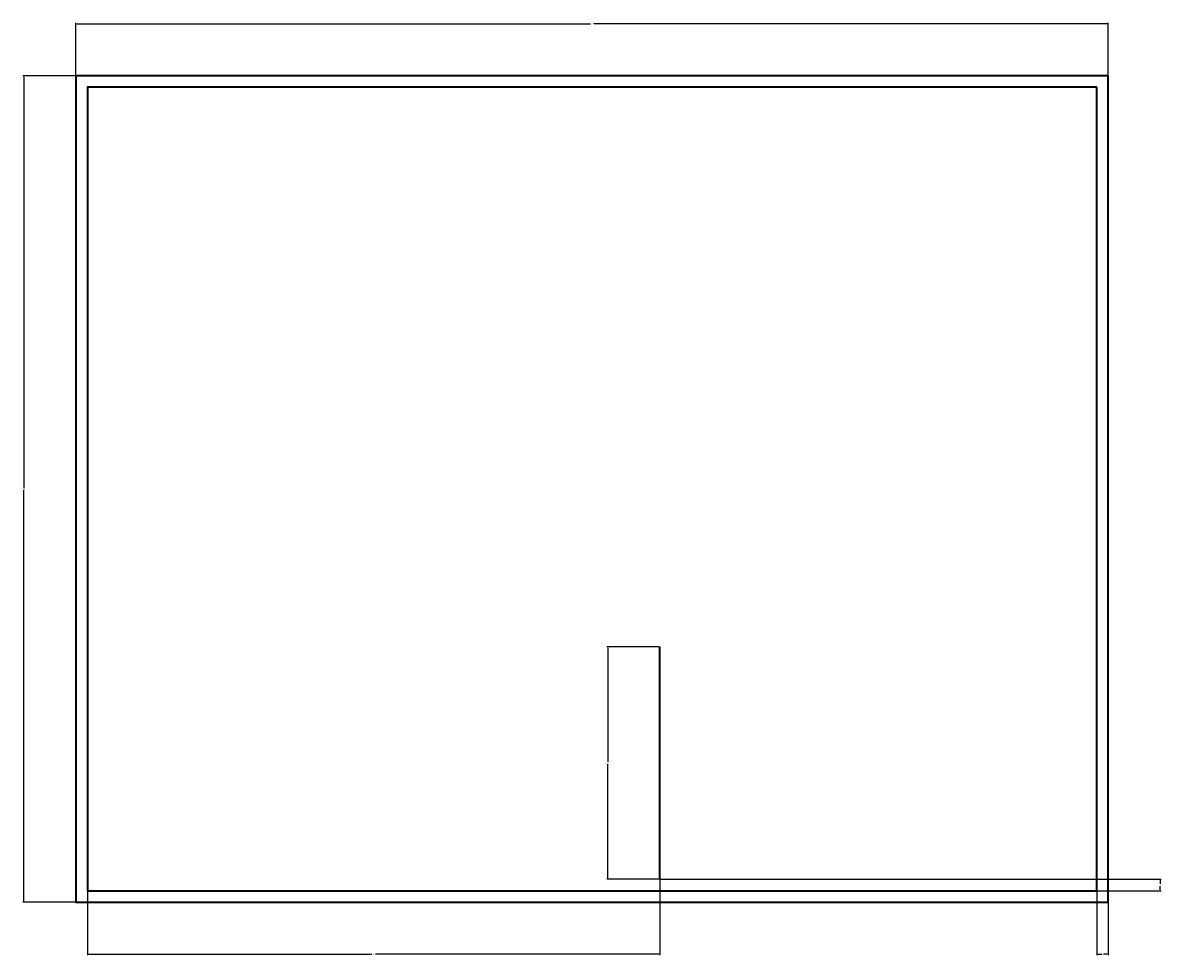
# Model space of a CAD drawing. Units: feet. Extents: x 1914 to 2338, y 2098 to 2528.
# Tile 3 of 3: x 1914 to 2112, y 2365 to 2528. Entities that reach past the tile are written whole.
import ezdxf

# ---------------------------------------------------------------- set-up
doc = ezdxf.new("R2010")
doc.units = ezdxf.units.FT
doc.layers.add('A-ANNO-DIMS', color=2, linetype='Continuous', lineweight=18)
doc.layers.add('A-ROOF', color=7, linetype='Continuous', lineweight=35)
doc.styles.get("Standard").update_dxf_attribs({"font": 'arial.ttf'})
doc.dimstyles.get("Standard").update_dxf_attribs({"dimtxt": 0.18, "dimasz": 0.18, "dimexe": 0.18, "dimexo": 0.0625, "dimgap": 0.09, "dimtad": 0, "dimtih": 1, "dimtoh": 1, "dimdec": 1, "dimzin": 0, "dimdsep": 46, "dimlunit": 3, "dimtxsty": 'Standard', "dimcen": 0.09, "dimadec": 0, "dimazin": 0, "dimtfac": 1, "dimtdec": 1, "dimtofl": 0, "dimtmove": 0, "dimatfit": 3, "dimfxl": 1, "dimtolj": 1, "dimtzin": 0, "dimarcsym": 0})

# ---------------------------------------------------------------- blocks, each defined once
blk = doc.blocks.new('*D54')
at = {"layer": 'A-ANNO-DIMS', "color": 0, "lineweight": -2, "transparency": 16777216}
for p, q in [((1922.85, 2518.49), (1922.85, 2527.66)), ((1923.03, 2527.48), (2012.57, 2527.48)), ((2102.67, 2527.48), (2013.13, 2527.48)), ((2102.85, 2518.49), (2102.85, 2527.66))]:
    blk.add_line(p, q, dxfattribs=at)
at = {"layer": 'A-ANNO-DIMS', "color": 0, "transparency": 16777216}
for points in [[(1923.03, 2527.51), (1923.03, 2527.45), (1922.85, 2527.48)], [(2102.67, 2527.51), (2102.67, 2527.45), (2102.85, 2527.48)]]:
    blk.add_solid(points, dxfattribs=at)
at = {"layer": 'Defpoints', "color": 0, "transparency": 16777216}
for p in [(2102.85, 2527.48), (1922.85, 2518.43), (2102.85, 2518.43)]:
    blk.add_point(p, dxfattribs=at)
at = {"layer": 'A-ANNO-DIMS', "color": 0, "transparency": 16777216, "insert": (2012.85, 2527.48), "char_height": 0.18, "attachment_point": 5}
blk.add_mtext('\\A1;180', dxfattribs=at)
blk = doc.blocks.new('*D55')
at = {"layer": 'A-ANNO-DIMS', "color": 0, "lineweight": -2, "transparency": 16777216}
for p, q in [((1922.78, 2518.43), (1913.61, 2518.43)), ((1913.79, 2518.25), (1913.79, 2446.61)), ((1913.79, 2374.61), (1913.79, 2446.25)), ((1922.78, 2374.43), (1913.61, 2374.43))]:
    blk.add_line(p, q, dxfattribs=at)
at = {"layer": 'A-ANNO-DIMS', "color": 0, "transparency": 16777216}
for points in [[(1913.76, 2518.25), (1913.82, 2518.25), (1913.79, 2518.43)], [(1913.76, 2374.61), (1913.82, 2374.61), (1913.79, 2374.43)]]:
    blk.add_solid(points, dxfattribs=at)
at = {"layer": 'Defpoints', "color": 0, "transparency": 16777216}
for p in [(1913.79, 2518.43), (1922.85, 2518.43), (1922.85, 2374.43)]:
    blk.add_point(p, dxfattribs=at)
at = {"layer": 'A-ANNO-DIMS', "color": 0, "transparency": 16777216, "insert": (1913.79, 2446.43), "char_height": 0.18, "attachment_point": 5}
blk.add_mtext('\\A1;144', dxfattribs=at)
blk = doc.blocks.new('*D56')
at = {"layer": 'A-ANNO-DIMS', "color": 0, "lineweight": -2, "transparency": 16777216}
for p, q in [((2024.64, 2378.36), (2024.64, 2365.19)), ((1924.85, 2376.36), (1924.85, 2365.19)), ((1925.03, 2365.37), (1974.42, 2365.37)), ((2024.46, 2365.37), (1975.07, 2365.37))]:
    blk.add_line(p, q, dxfattribs=at)
at = {"layer": 'A-ANNO-DIMS', "color": 0, "transparency": 16777216}
for points in [[(1925.03, 2365.4), (1925.03, 2365.34), (1924.85, 2365.37)], [(2024.46, 2365.4), (2024.46, 2365.34), (2024.64, 2365.37)]]:
    blk.add_solid(points, dxfattribs=at)
at = {"layer": 'Defpoints', "color": 0, "transparency": 16777216}
for p in [(2024.64, 2378.43), (1924.85, 2376.43), (2024.64, 2365.37)]:
    blk.add_point(p, dxfattribs=at)
at = {"layer": 'A-ANNO-DIMS', "color": 0, "transparency": 16777216, "insert": (1974.74, 2365.37), "char_height": 0.18, "attachment_point": 5}
blk.add_mtext('\\A1;99.8', dxfattribs=at)
blk = doc.blocks.new('*D57')
at = {"layer": 'A-ANNO-DIMS', "color": 0, "lineweight": -2, "transparency": 16777216}
for p, q in [((2024.58, 2418.93), (2015.41, 2418.93)), ((2015.59, 2418.75), (2015.59, 2398.86)), ((2015.59, 2378.61), (2015.59, 2398.49)), ((2024.58, 2378.43), (2015.41, 2378.43))]:
    blk.add_line(p, q, dxfattribs=at)
at = {"layer": 'A-ANNO-DIMS', "color": 0, "transparency": 16777216}
for points in [[(2015.56, 2418.75), (2015.62, 2418.75), (2015.59, 2418.93)], [(2015.56, 2378.61), (2015.62, 2378.61), (2015.59, 2378.43)]]:
    blk.add_solid(points, dxfattribs=at)
at = {"layer": 'Defpoints', "color": 0, "transparency": 16777216}
for p in [(2015.59, 2418.93), (2024.64, 2418.93), (2024.64, 2378.43)]:
    blk.add_point(p, dxfattribs=at)
at = {"layer": 'A-ANNO-DIMS', "color": 0, "transparency": 16777216, "insert": (2015.59, 2398.68), "char_height": 0.18, "attachment_point": 5}
blk.add_mtext('\\A1;40.5', dxfattribs=at)
blk = doc.blocks.new('*D58')
at = {"layer": 'A-ANNO-DIMS', "color": 0, "lineweight": -2, "transparency": 16777216}
for p, q in [((2100.85, 2376.36), (2100.85, 2365.19)), ((2102.85, 2374.36), (2102.85, 2365.19)), ((2101.03, 2365.37), (2101.7, 2365.37)), ((2102.67, 2365.37), (2102, 2365.37))]:
    blk.add_line(p, q, dxfattribs=at)
at = {"layer": 'A-ANNO-DIMS', "color": 0, "transparency": 16777216}
for points in [[(2101.03, 2365.4), (2101.03, 2365.34), (2100.85, 2365.37)], [(2102.67, 2365.4), (2102.67, 2365.34), (2102.85, 2365.37)]]:
    blk.add_solid(points, dxfattribs=at)
at = {"layer": 'Defpoints', "color": 0, "transparency": 16777216}
for p in [(2100.85, 2376.43), (2102.85, 2374.43), (2102.85, 2365.37)]:
    blk.add_point(p, dxfattribs=at)
at = {"layer": 'A-ANNO-DIMS', "color": 0, "transparency": 16777216, "insert": (2101.85, 2365.37), "char_height": 0.18, "attachment_point": 5}
blk.add_mtext('\\A1;2', dxfattribs=at)
blk = doc.blocks.new('*D59')
at = {"layer": 'A-ANNO-DIMS', "color": 0, "lineweight": -2, "transparency": 16777216}
for p, q in [((2024.71, 2378.43), (2112.08, 2378.43)), ((2111.9, 2378.25), (2111.9, 2377.61)), ((2100.91, 2376.43), (2112.08, 2376.43)), ((2111.9, 2376.61), (2111.9, 2377.25))]:
    blk.add_line(p, q, dxfattribs=at)
at = {"layer": 'A-ANNO-DIMS', "color": 0, "transparency": 16777216}
for points in [[(2111.87, 2378.25), (2111.93, 2378.25), (2111.9, 2378.43)], [(2111.87, 2376.61), (2111.93, 2376.61), (2111.9, 2376.43)]]:
    blk.add_solid(points, dxfattribs=at)
at = {"layer": 'Defpoints', "color": 0, "transparency": 16777216}
for p in [(2024.64, 2378.43), (2111.9, 2378.43), (2100.85, 2376.43)]:
    blk.add_point(p, dxfattribs=at)
at = {"layer": 'A-ANNO-DIMS', "color": 0, "transparency": 16777216, "insert": (2111.9, 2377.43), "char_height": 0.18, "attachment_point": 5}
blk.add_mtext('\\A1;2', dxfattribs=at)

msp = doc.modelspace()

# ---------------------------------------------------------------- linework, layer by layer
at = {"layer": 'A-ROOF'}
msp.add_line((2024.6434, 2378.4255, 246), (2024.6434, 2418.9255, 246), dxfattribs=at)
at = {"layer": 'A-ROOF', "elevation": 288}
for points in [[(2102.8458, 2518.4255), (1922.8458, 2518.4255), (1922.8458, 2374.4255), (2102.8458, 2374.4255)], [(2100.8458, 2516.4255), (1924.8458, 2516.4255), (1924.8458, 2376.4255), (2100.8458, 2376.4255)]]:
    msp.add_lwpolyline(points, close=True, dxfattribs=at)

# ---------------------------------------------------------------- dimensions: what is measured, and where the dimension line sits
at = {"layer": 'A-ANNO-DIMS'}
for base, p1, p2, override, picture, middle in [((2102.8458, 2527.4806), (1922.8458, 2518.4255), (2102.8458, 2518.4255), {"dimdec": 0, "dimlfac": 1, "dimrnd": 0, "dimzin": 0, "dimdsep": 46, "dimlunit": 2}, '*D54', (2012.8458, 2527.4806)), ((2024.6434, 2365.3706), (1924.8458, 2376.4255), (2024.6434, 2378.4255), {"dimdec": 1, "dimlfac": 1, "dimrnd": 0, "dimzin": 0, "dimdsep": 46, "dimlunit": 2}, '*D56', (1974.7446, 2365.3706)), ((2102.8458, 2365.3706), (2100.8458, 2376.4255), (2102.8458, 2374.4255), {"dimdec": 0, "dimlfac": 1, "dimrnd": 0, "dimzin": 0, "dimdsep": 46, "dimlunit": 2}, '*D58', (2101.8458, 2365.3706))]:
    dim = msp.add_linear_dim(base=base, p1=p1, p2=p2, dimstyle='Standard', override=override, dxfattribs=at)
    dim.commit()
    dim.dimension.update_dxf_attribs({"geometry": picture, "text_midpoint": middle})
for base, p1, p2, override, picture, middle in [((1913.7908, 2518.4255), (1922.8458, 2374.4255), (1922.8458, 2518.4255), {"dimdec": 0, "dimlfac": 1, "dimrnd": 0, "dimzin": 0, "dimdsep": 46, "dimlunit": 2}, '*D55', (1913.7908, 2446.4255)), ((2015.5884, 2418.9255), (2024.6434, 2378.4255), (2024.6434, 2418.9255), {"dimdec": 1, "dimlfac": 1, "dimrnd": 0, "dimzin": 0, "dimdsep": 46, "dimlunit": 2}, '*D57', (2015.5884, 2398.6755)), ((2111.9008, 2378.4255), (2100.8458, 2376.4255), (2024.6434, 2378.4255), {"dimdec": 0, "dimlfac": 1, "dimrnd": 0, "dimzin": 0, "dimdsep": 46, "dimlunit": 2}, '*D59', (2111.9008, 2377.4255))]:
    dim = msp.add_linear_dim(base=base, p1=p1, p2=p2, angle=90, dimstyle='Standard', override=override, dxfattribs=at)
    dim.commit()
    dim.dimension.update_dxf_attribs({"geometry": picture, "text_midpoint": middle})

doc.saveas('drawing.dxf')
